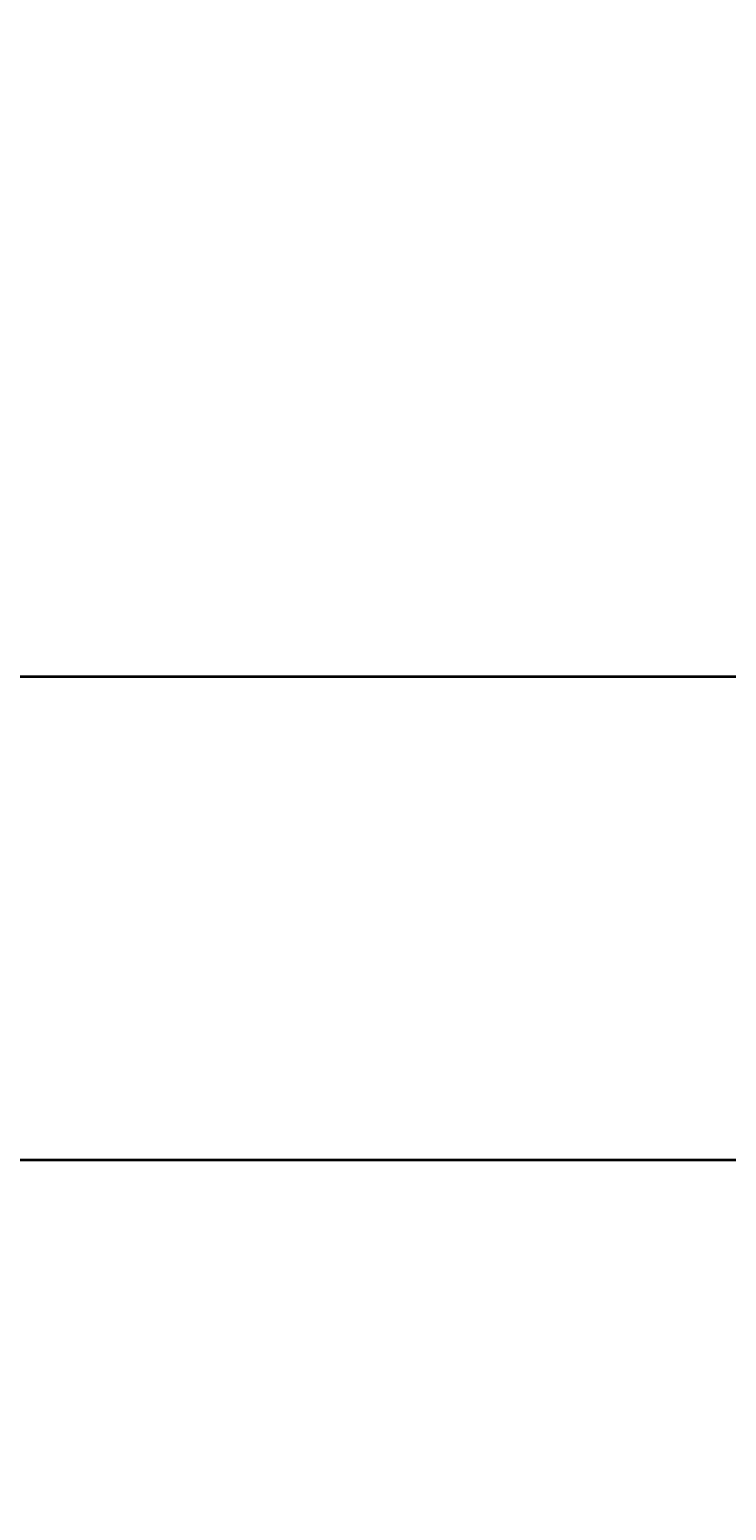
# Model space of a CAD drawing. Units: millimetres. Extents: x 27017497 to 27018854, y 7058029 to 7059154.
# Tile 65 of 91: x 27018342 to 27018355, y 7058126 to 7058154. Entities that reach past the tile are written whole.
import ezdxf

# ---------------------------------------------------------------- set-up
doc = ezdxf.new("R2010")
doc.units = ezdxf.units.MM
for name, color, linetype, lineweight in [('A-ANNO-DIMS', 2, 'Continuous', 18), ('A-FLOR-CASE-PATT', 44, 'Continuous', 13), ('A-WALL', 7, 'Continuous', 35)]:
    doc.layers.add(name, color=color, linetype=linetype, lineweight=lineweight)
doc.styles.get("Standard").update_dxf_attribs({"font": 'arial.ttf'})
doc.dimstyles.get("Standard").update_dxf_attribs({"dimtxt": 0.18, "dimasz": 0.18, "dimexe": 0.18, "dimexo": 0.0625, "dimgap": 0.09, "dimtad": 0, "dimtih": 1, "dimtoh": 1, "dimdec": 4, "dimzin": 0, "dimdsep": 46, "dimtxsty": 'Standard', "dimcen": 0.09, "dimadec": 0, "dimazin": 0, "dimtfac": 1, "dimtdec": 4, "dimtofl": 0, "dimtmove": 0, "dimatfit": 3, "dimfxl": 1, "dimtolj": 1, "dimtzin": 0, "dimarcsym": 0})

# ---------------------------------------------------------------- blocks, each defined once
blk = doc.blocks.new('*D47')
at = {"layer": 'A-ANNO-DIMS', "color": 0, "lineweight": -2, "transparency": 16777216}
for p, q in [((27017561.166, 7058294.35), (27017561.166, 7058028.6)), ((27018790.606, 7058294.35), (27018790.606, 7058028.6)), ((27017561.346, 7058028.78), (27018175.431, 7058028.78)), ((27018790.426, 7058028.78), (27018176.341, 7058028.78))]:
    blk.add_line(p, q, dxfattribs=at)
at = {"layer": 'A-ANNO-DIMS', "color": 0, "transparency": 16777216}
for points in [[(27017561.346, 7058028.81), (27017561.346, 7058028.75), (27017561.166, 7058028.78)], [(27018790.426, 7058028.81), (27018790.426, 7058028.75), (27018790.606, 7058028.78)]]:
    blk.add_solid(points, dxfattribs=at)
at = {"layer": 'Defpoints', "color": 0, "transparency": 16777216}
for p in [(27017561.166, 7058294.412), (27018790.606, 7058294.412), (27018790.606, 7058028.78)]:
    blk.add_point(p, dxfattribs=at)
at = {"layer": 'A-ANNO-DIMS', "color": 0, "transparency": 16777216, "insert": (27018175.886, 7058028.78), "char_height": 0.18, "attachment_point": 5}
blk.add_mtext('\\A1;1229.4', dxfattribs=at)
blk = doc.blocks.new('*D48')
at = {"layer": 'A-ANNO-DIMS', "color": 0, "lineweight": -2, "transparency": 16777216}
for p, q in [((27018463.498, 7058622.912), (27017497.536, 7058622.912)), ((27017497.716, 7058622.732), (27017497.716, 7058357.753)), ((27017497.716, 7058092.41), (27017497.716, 7058357.389)), ((27018555.129, 7058092.23), (27017497.536, 7058092.23))]:
    blk.add_line(p, q, dxfattribs=at)
at = {"layer": 'A-ANNO-DIMS', "color": 0, "transparency": 16777216}
for points in [[(27017497.686, 7058622.732), (27017497.746, 7058622.732), (27017497.716, 7058622.912)], [(27017497.686, 7058092.41), (27017497.746, 7058092.41), (27017497.716, 7058092.23)]]:
    blk.add_solid(points, dxfattribs=at)
at = {"layer": 'Defpoints', "color": 0, "transparency": 16777216}
for p in [(27018463.561, 7058622.912), (27017497.716, 7058092.23), (27018555.192, 7058092.23)]:
    blk.add_point(p, dxfattribs=at)
at = {"layer": 'A-ANNO-DIMS', "color": 0, "transparency": 16777216, "insert": (27017497.716, 7058357.571), "char_height": 0.18, "attachment_point": 5}
blk.add_mtext('\\A1;530.7', dxfattribs=at)

msp = doc.modelspace()

# ---------------------------------------------------------------- hatches: boundary and pattern name
at = {"layer": 'A-FLOR-CASE-PATT'}
h = msp.add_hatch(color=256, dxfattribs=at)
h.dxf.hatch_style = 1
edge = h.paths.add_edge_path()
edge.add_line((27018341.343, 7058207.055), (27018330.837, 7058207.055))
edge.add_line((27018330.837, 7058207.055), (27018330.837, 7058203.02))
edge.add_line((27018330.837, 7058203.02), (27018338.424, 7058203.02))
edge.add_ellipse((27018338.23, 7058202.551), major_axis=(0.528, 0), ratio=0.888892, start_angle=0, end_angle=90, ccw=False)
edge.add_line((27018338.758, 7058202.551), (27018338.758, 7058202.238))
edge.add_line((27018338.758, 7058202.238), (27018330.837, 7058201.488))
edge.add_line((27018330.837, 7058201.488), (27018330.837, 7058199.747))
edge.add_line((27018330.837, 7058199.747), (27018338.424, 7058199.747))
edge.add_ellipse((27018338.23, 7058199.277), major_axis=(0.528, 0), ratio=0.888892, start_angle=0, end_angle=90, ccw=False)
edge.add_line((27018338.758, 7058199.277), (27018338.758, 7058198.964))
edge.add_line((27018338.758, 7058198.964), (27018330.837, 7058198.215))
edge.add_line((27018330.837, 7058198.215), (27018330.837, 7058193.415))
edge.add_line((27018330.837, 7058193.415), (27018338.284, 7058190.704))
edge.add_ellipse((27018337.942, 7058190.329), major_axis=(0.496, -0.181), ratio=0.888892, start_angle=0, end_angle=90, ccw=False)
edge.add_line((27018338.439, 7058190.148), (27018338.331, 7058189.854))
edge.add_line((27018338.331, 7058189.854), (27018330.837, 7058191.806))
edge.add_line((27018330.837, 7058191.806), (27018330.837, 7058188.22))
edge.add_line((27018330.837, 7058188.22), (27018338.424, 7058188.22))
edge.add_ellipse((27018338.23, 7058187.75), major_axis=(0.528, 0), ratio=0.888892, start_angle=0, end_angle=90, ccw=False)
edge.add_line((27018338.758, 7058187.75), (27018338.758, 7058187.437))
edge.add_line((27018338.758, 7058187.437), (27018330.837, 7058186.688))
edge.add_line((27018330.837, 7058186.688), (27018330.837, 7058181.982))
edge.add_line((27018330.837, 7058181.982), (27018338.424, 7058181.982))
edge.add_ellipse((27018338.23, 7058181.513), major_axis=(0.528, 0), ratio=0.888892, start_angle=0, end_angle=90, ccw=False)
edge.add_line((27018338.758, 7058181.513), (27018338.758, 7058181.199))
edge.add_line((27018338.758, 7058181.199), (27018330.837, 7058180.45))
edge.add_line((27018330.837, 7058180.45), (27018330.837, 7058178.709))
edge.add_line((27018330.837, 7058178.709), (27018338.424, 7058178.709))
edge.add_ellipse((27018338.23, 7058178.239), major_axis=(0.528, 0), ratio=0.888892, start_angle=0, end_angle=90, ccw=False)
edge.add_line((27018338.758, 7058178.239), (27018338.758, 7058177.926))
edge.add_line((27018338.758, 7058177.926), (27018330.837, 7058177.177))
edge.add_line((27018330.837, 7058177.177), (27018330.837, 7058173.878))
edge.add_line((27018330.837, 7058173.878), (27018338.284, 7058171.167))
edge.add_ellipse((27018337.942, 7058170.792), major_axis=(0.496, -0.181), ratio=0.888892, start_angle=0, end_angle=90, ccw=False)
edge.add_line((27018338.439, 7058170.611), (27018338.331, 7058170.317))
edge.add_line((27018338.331, 7058170.317), (27018330.837, 7058172.269))
edge.add_line((27018330.837, 7058172.269), (27018330.837, 7058168.293))
edge.add_line((27018330.837, 7058168.293), (27018338.424, 7058168.293))
edge.add_ellipse((27018338.23, 7058167.824), major_axis=(0.528, 0), ratio=0.888892, start_angle=0, end_angle=90, ccw=False)
edge.add_line((27018338.758, 7058167.824), (27018338.758, 7058167.511))
edge.add_line((27018338.758, 7058167.511), (27018330.837, 7058166.762))
edge.add_line((27018330.837, 7058166.762), (27018330.837, 7058160.389))
edge.add_line((27018330.837, 7058160.389), (27018338.424, 7058160.389))
edge.add_ellipse((27018338.23, 7058159.92), major_axis=(0.528, 0), ratio=0.888892, start_angle=0, end_angle=90, ccw=False)
edge.add_line((27018338.758, 7058159.92), (27018338.758, 7058159.607))
edge.add_line((27018338.758, 7058159.607), (27018330.837, 7058158.858))
edge.add_line((27018330.837, 7058158.858), (27018330.837, 7058157.116))
edge.add_line((27018330.837, 7058157.116), (27018338.424, 7058157.116))
edge.add_ellipse((27018338.23, 7058156.647), major_axis=(0.528, 0), ratio=0.888892, start_angle=0, end_angle=90, ccw=False)
edge.add_line((27018338.758, 7058156.647), (27018338.758, 7058156.334))
edge.add_line((27018338.758, 7058156.334), (27018330.837, 7058155.585))
edge.add_line((27018330.837, 7058155.585), (27018330.837, 7058150.784))
edge.add_line((27018330.837, 7058150.784), (27018338.284, 7058148.073))
edge.add_ellipse((27018337.942, 7058147.698), major_axis=(0.496, -0.181), ratio=0.888892, start_angle=0, end_angle=90, ccw=False)
edge.add_line((27018338.439, 7058147.517), (27018338.331, 7058147.223))
edge.add_line((27018338.331, 7058147.223), (27018330.837, 7058149.175))
edge.add_line((27018330.837, 7058149.175), (27018330.837, 7058145.589))
edge.add_line((27018330.837, 7058145.589), (27018338.424, 7058145.589))
edge.add_ellipse((27018338.23, 7058145.119), major_axis=(0.528, 0), ratio=0.888892, start_angle=0, end_angle=90, ccw=False)
edge.add_line((27018338.758, 7058145.119), (27018338.758, 7058144.806))
edge.add_line((27018338.758, 7058144.806), (27018330.837, 7058144.057))
edge.add_line((27018330.837, 7058144.057), (27018330.837, 7058141.912))
edge.add_line((27018330.837, 7058141.912), (27018341.343, 7058141.912))
edge.add_line((27018341.343, 7058141.912), (27018341.343, 7058207.055))
edge = h.paths.add_edge_path()
edge.add_line((27018330.112, 7058207.055), (27018319.606, 7058207.055))
edge.add_line((27018319.606, 7058207.055), (27018319.606, 7058141.912))
edge.add_line((27018319.606, 7058141.912), (27018330.112, 7058141.912))
edge.add_line((27018330.112, 7058141.912), (27018330.112, 7058144.024))
edge.add_line((27018330.112, 7058144.024), (27018322.543, 7058144.024))
edge.add_ellipse((27018322.736, 7058144.493), major_axis=(0.528, 0), ratio=0.888892, start_angle=180, end_angle=270, ccw=False)
edge.add_line((27018322.208, 7058144.493), (27018322.208, 7058145.291))
edge.add_ellipse((27018322.736, 7058145.119), major_axis=(0.528, 0), ratio=0.888892, start_angle=90, end_angle=180, ccw=False)
edge.add_line((27018322.736, 7058145.589), (27018330.112, 7058145.589))
edge.add_line((27018330.112, 7058145.589), (27018330.112, 7058149.382))
edge.add_line((27018330.112, 7058149.382), (27018322.826, 7058152.034))
edge.add_ellipse((27018323.168, 7058152.409), major_axis=(0.496, -0.181), ratio=0.888892, start_angle=180, end_angle=270, ccw=False)
edge.add_line((27018322.672, 7058152.59), (27018322.945, 7058153.34))
edge.add_ellipse((27018323.382, 7058152.997), major_axis=(0.496, -0.181), ratio=0.888892, start_angle=90, end_angle=180, ccw=False)
edge.add_line((27018323.543, 7058153.439), (27018330.112, 7058151.048))
edge.add_line((27018330.112, 7058151.048), (27018330.112, 7058155.551))
edge.add_line((27018330.112, 7058155.551), (27018322.543, 7058155.551))
edge.add_ellipse((27018322.736, 7058156.021), major_axis=(0.528, 0), ratio=0.888892, start_angle=180, end_angle=270, ccw=False)
edge.add_line((27018322.208, 7058156.021), (27018322.208, 7058156.819))
edge.add_ellipse((27018322.736, 7058156.647), major_axis=(0.528, 0), ratio=0.888892, start_angle=90, end_angle=180, ccw=False)
edge.add_line((27018322.736, 7058157.116), (27018330.112, 7058157.116))
edge.add_line((27018330.112, 7058157.116), (27018330.112, 7058158.824))
edge.add_line((27018330.112, 7058158.824), (27018322.543, 7058158.824))
edge.add_ellipse((27018322.736, 7058159.294), major_axis=(0.528, 0), ratio=0.888892, start_angle=180, end_angle=270, ccw=False)
edge.add_line((27018322.208, 7058159.294), (27018322.208, 7058160.092))
edge.add_ellipse((27018322.736, 7058159.92), major_axis=(0.528, 0), ratio=0.888892, start_angle=90, end_angle=180, ccw=False)
edge.add_line((27018322.736, 7058160.389), (27018330.112, 7058160.389))
edge.add_line((27018330.112, 7058160.389), (27018330.112, 7058166.728))
edge.add_line((27018330.112, 7058166.728), (27018322.543, 7058166.728))
edge.add_ellipse((27018322.736, 7058167.198), major_axis=(0.528, 0), ratio=0.888892, start_angle=180, end_angle=270, ccw=False)
edge.add_line((27018322.208, 7058167.198), (27018322.208, 7058167.996))
edge.add_ellipse((27018322.736, 7058167.824), major_axis=(0.528, 0), ratio=0.888892, start_angle=90, end_angle=180, ccw=False)
edge.add_line((27018322.736, 7058168.293), (27018330.112, 7058168.293))
edge.add_line((27018330.112, 7058168.293), (27018330.112, 7058172.476))
edge.add_line((27018330.112, 7058172.476), (27018322.826, 7058175.128))
edge.add_ellipse((27018323.168, 7058175.503), major_axis=(0.496, -0.181), ratio=0.888892, start_angle=180, end_angle=270, ccw=False)
edge.add_line((27018322.672, 7058175.684), (27018322.945, 7058176.433))
edge.add_ellipse((27018323.382, 7058176.091), major_axis=(0.496, -0.181), ratio=0.888892, start_angle=90, end_angle=180, ccw=False)
edge.add_line((27018323.543, 7058176.533), (27018330.112, 7058174.142))
edge.add_line((27018330.112, 7058174.142), (27018330.112, 7058177.144))
edge.add_line((27018330.112, 7058177.144), (27018322.543, 7058177.144))
edge.add_ellipse((27018322.736, 7058177.613), major_axis=(0.528, 0), ratio=0.888892, start_angle=180, end_angle=270, ccw=False)
edge.add_line((27018322.208, 7058177.613), (27018322.208, 7058178.411))
edge.add_ellipse((27018322.736, 7058178.239), major_axis=(0.528, 0), ratio=0.888892, start_angle=90, end_angle=180, ccw=False)
edge.add_line((27018322.736, 7058178.709), (27018330.112, 7058178.709))
edge.add_line((27018330.112, 7058178.709), (27018330.112, 7058180.417))
edge.add_line((27018330.112, 7058180.417), (27018322.543, 7058180.417))
edge.add_ellipse((27018322.736, 7058180.886), major_axis=(0.528, 0), ratio=0.888892, start_angle=180, end_angle=270, ccw=False)
edge.add_line((27018322.208, 7058180.886), (27018322.208, 7058181.684))
edge.add_ellipse((27018322.736, 7058181.513), major_axis=(0.528, 0), ratio=0.888892, start_angle=90, end_angle=180, ccw=False)
edge.add_line((27018322.736, 7058181.982), (27018330.112, 7058181.982))
edge.add_line((27018330.112, 7058181.982), (27018330.112, 7058186.655))
edge.add_line((27018330.112, 7058186.655), (27018322.543, 7058186.655))
edge.add_ellipse((27018322.736, 7058187.124), major_axis=(0.528, 0), ratio=0.888892, start_angle=180, end_angle=270, ccw=False)
edge.add_line((27018322.208, 7058187.124), (27018322.208, 7058187.922))
edge.add_ellipse((27018322.736, 7058187.75), major_axis=(0.528, 0), ratio=0.888892, start_angle=90, end_angle=180, ccw=False)
edge.add_line((27018322.736, 7058188.22), (27018330.112, 7058188.22))
edge.add_line((27018330.112, 7058188.22), (27018330.112, 7058192.013))
edge.add_line((27018330.112, 7058192.013), (27018322.826, 7058194.665))
edge.add_ellipse((27018323.168, 7058195.04), major_axis=(0.496, -0.181), ratio=0.888892, start_angle=180, end_angle=270, ccw=False)
edge.add_line((27018322.672, 7058195.22), (27018322.945, 7058195.97))
edge.add_ellipse((27018323.382, 7058195.628), major_axis=(0.496, -0.181), ratio=0.888892, start_angle=90, end_angle=180, ccw=False)
edge.add_line((27018323.543, 7058196.069), (27018330.112, 7058193.678))
edge.add_line((27018330.112, 7058193.678), (27018330.112, 7058198.182))
edge.add_line((27018330.112, 7058198.182), (27018322.543, 7058198.182))
edge.add_ellipse((27018322.736, 7058198.651), major_axis=(0.528, 0), ratio=0.888892, start_angle=180, end_angle=270, ccw=False)
edge.add_line((27018322.208, 7058198.651), (27018322.208, 7058199.449))
edge.add_ellipse((27018322.736, 7058199.277), major_axis=(0.528, 0), ratio=0.888892, start_angle=90, end_angle=180, ccw=False)
edge.add_line((27018322.736, 7058199.747), (27018330.112, 7058199.747))
edge.add_line((27018330.112, 7058199.747), (27018330.112, 7058201.455))
edge.add_line((27018330.112, 7058201.455), (27018322.543, 7058201.455))
edge.add_ellipse((27018322.736, 7058201.924), major_axis=(0.528, 0), ratio=0.888892, start_angle=180, end_angle=270, ccw=False)
edge.add_line((27018322.208, 7058201.924), (27018322.208, 7058202.722))
edge.add_ellipse((27018322.736, 7058202.551), major_axis=(0.528, 0), ratio=0.888892, start_angle=90, end_angle=180, ccw=False)
edge.add_line((27018322.736, 7058203.02), (27018330.112, 7058203.02))
edge.add_line((27018330.112, 7058203.02), (27018330.112, 7058207.055))
h.paths.add_polyline_path([(27018341.31, 7058294.412), (27018319.606, 7058294.412), (27018319.606, 7058207.1), (27018341.31, 7058207.1)])
h.paths.add_polyline_path([(27018354.358, 7058255.592), (27018354.358, 7058256.057, -0.414214), (27018354.869, 7058256.569), (27018346.477, 7058256.569, -0.414214), (27018345.197, 7058257.848), (27018345.197, 7058259.128, -0.414214), (27018346.477, 7058260.407), (27018343.868, 7058260.407, 0.290979), (27018341.551, 7058258.934), (27018341.551, 7058242.534, 0.290979), (27018343.868, 7058241.06), (27018346.477, 7058241.06, -0.414214), (27018345.197, 7058242.34), (27018345.197, 7058243.619, -0.414214), (27018346.477, 7058244.899), (27018353.078, 7058244.899, 0.414214), (27018354.358, 7058246.178)])
h.paths.add_polyline_path([(27018356.917, 7058260.407), (27018346.477, 7058260.407, 0.414214), (27018345.197, 7058259.128), (27018345.197, 7058257.848, 0.414214), (27018346.477, 7058256.569), (27018355.637, 7058256.569), (27018355.637, 7058244.899), (27018346.477, 7058244.899, 0.414214), (27018345.197, 7058243.619), (27018345.197, 7058242.34, 0.414214), (27018346.477, 7058241.06), (27018356.917, 7058241.06, 0.414214), (27018359.476, 7058243.619), (27018359.476, 7058257.848, 0.414214)])
h.paths.add_polyline_path([(27018355.637, 7058252.362), (27018355.637, 7058256.057, 0.490314), (27018354.997, 7058256.553, 0.490314), (27018354.358, 7058256.057), (27018354.358, 7058255.592), (27018354.358, 7058245.411, 0.490314), (27018354.997, 7058244.915, 0.490314), (27018355.637, 7058245.411)], flags=17)

# ---------------------------------------------------------------- linework, layer by layer
at = {"layer": 'A-WALL'}
for p, q in [((27018468.106, 7058141.912), (27018319.606, 7058141.912)), ((27018468.106, 7058132.912), (27018310.606, 7058132.912))]:
    msp.add_line(p, q, dxfattribs=at)

# ---------------------------------------------------------------- dimensions: what is measured, and where the dimension line sits
at = {"layer": 'A-ANNO-DIMS'}
dim = msp.add_linear_dim(base=(27017497.716, 7058092.23), p1=(27018463.561, 7058622.912), p2=(27018555.192, 7058092.23), angle=90, dimstyle='Standard', override={"dimdec": 1, "dimlfac": 1, "dimrnd": 0, "dimzin": 0, "dimdsep": 46, "dimlunit": 2}, dxfattribs=at)
dim.commit()
dim.dimension.update_dxf_attribs({"geometry": '*D48', "text_midpoint": (27017497.716, 7058357.571)})
dim = msp.add_linear_dim(base=(27018790.606, 7058028.78), p1=(27017561.166, 7058294.412), p2=(27018790.606, 7058294.412), dimstyle='Standard', override={"dimdec": 1, "dimlfac": 1, "dimrnd": 0, "dimzin": 0, "dimdsep": 46, "dimlunit": 2}, dxfattribs=at)
dim.commit()
dim.dimension.update_dxf_attribs({"geometry": '*D47', "text_midpoint": (27018175.886, 7058028.78)})

doc.saveas('drawing.dxf')
